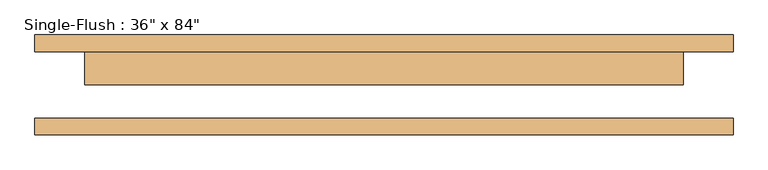
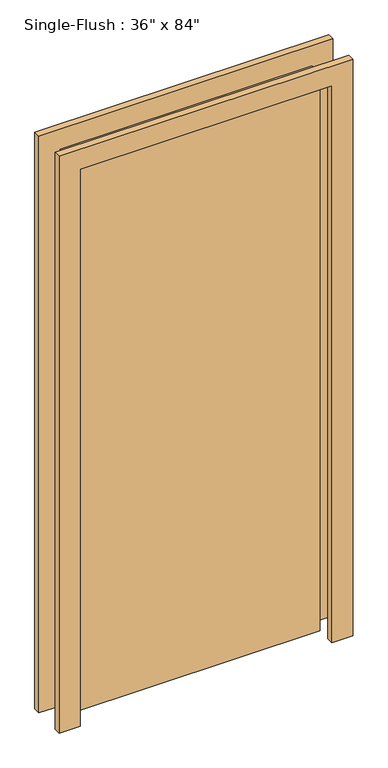
"""IFC4 building model written with IfcOpenShell, lengths in millimetres: door geometry."""

from ifc_helpers import new_model, si_unit, frame, origin, origin_with_axes, place, context, project, spatial, polyline, outline, extrude, source, transform, mapped, element, save


def door_048588e9(model_context):
    return source(origin(), model_context, "Body", "SweptSolid", [
        extrude(outline(polyline([(2209.8, -533.4), (0.0, -533.4), (0.0, -457.2), (2133.6, -457.2), (2133.6, 457.2), (0.0, 457.2), (0.0, 533.4), (2209.8, 533.4), (2209.8, -533.4)])), frame((0.0, 50.8, 0.0), z_axis=(0.0, 1.0, 0.0), x_axis=(0.0, 0.0, 1.0)), (0.0, 0.0, 1.0), 25.4),
        extrude(outline(polyline([(2209.8, 533.4), (2209.8, -533.4), (0.0, -533.4), (0.0, -457.2), (2133.6, -457.2), (2133.6, 457.2), (0.0, 457.2), (0.0, 533.4), (2209.8, 533.4)])), frame((0.0, -76.2, 0.0), z_axis=(0.0, 1.0, 0.0), x_axis=(0.0, 0.0, 1.0)), (0.0, 0.0, 1.0), 25.4),
        extrude(outline(polyline([(457.2, 0.0), (-457.2, 0.0), (-457.2, 50.8), (457.2, 50.8), (457.2, 0.0)])), origin_with_axes(), (0.0, 0.0, 1.0), 2133.6),
    ])


if __name__ == "__main__":
    model = new_model("IFC4")
    model_context = context("Model", 3, world=origin())
    ifc_project = project(units=[si_unit("LENGTHUNIT", "METRE", prefix="MILLI")], contexts=[model_context])
    site = spatial("IfcSite", under=ifc_project)
    building = spatial("IfcBuilding", under=site)
    placement = place(None, origin())
    door_shape = door_048588e9(model_context)
    element("IfcDoor", 1, ObjectType="Single-Flush : 36\" x 84\"", at=placement, inside=building, context=model_context, shape_type="MappedRepresentation", body=[
        mapped(door_shape, transform((0.0, 0.0, 0.0), x_axis=(1.0, 0.0, 0.0), y_axis=(0.0, 1.0, 0.0), z_axis=(0.0, 0.0, 1.0))),
    ])
    save(model, "model.ifc")

# Revit data of these elements
# Type "Single-Flush : 36\" x 84\""
#   Type Mark = "1"
#   Construction Type Id = "MDOOR"
#   Assembly Code = "C1020"
#   Analytic Construction = "Metal"
#   Thickness = 0' - 2"
#   Heat Transfer Coefficient (U) = 0.651978 BTU/(h·ft²·°F)
#   Height = 7' - 0"
#   Trim Projection Ext = 0' - 1"
#   Trim Projection Int = 0' - 1"
#   Trim Width = 0' - 3"
#   Width = 3' - 0"
#   Define Thermal Properties by = 1
#   Door Material = Door - Panel
#   Frame Material = Door - Frame
#   Visual Light Transmittance = 0
#   Solar Heat Gain Coefficient = 0
#   Function = (empty or 0)
#   Wall Closure = (empty or 0)
# Element 1 (IfcDoor, "Single-Flush : 36\" x 84\"")
#   Materials on its faces: "Door - Frame", "Door - Panel"
# Materials
#   "Door - Panel": class "Wood", colour RGB 210 159 95, transparency 0
#   "Door - Frame": colour RGB 118 70 51, transparency 0
